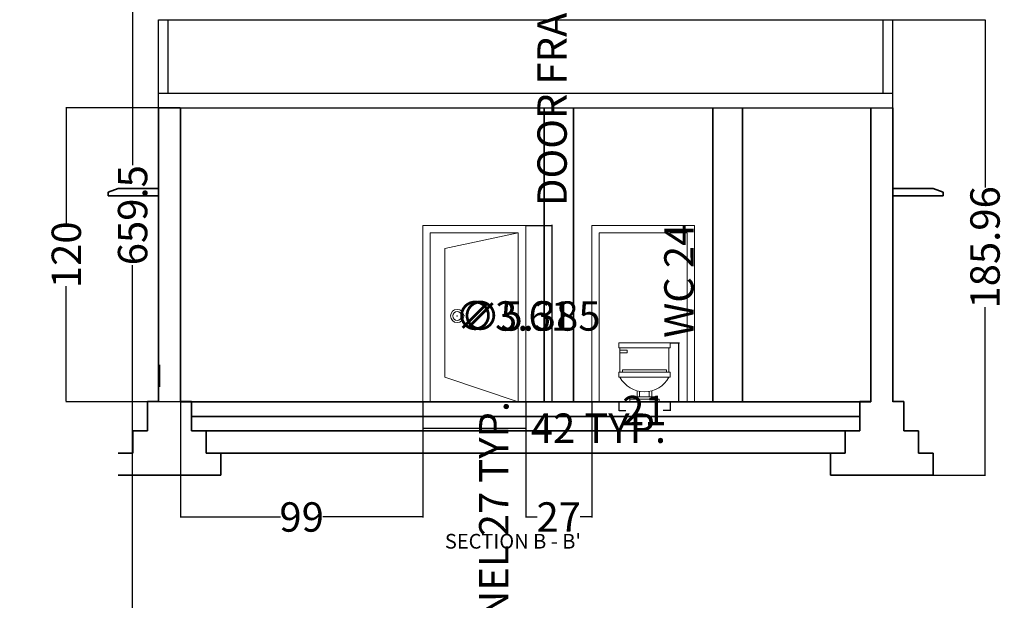
# Model space of a CAD drawing. Units: inches. Extents: x -101 to 786, y 26 to 880.
# Tile 8 of 9: x 379 to 781, y 295 to 532. Entities that reach past the tile are written whole.
import ezdxf

# ---------------------------------------------------------------- set-up
doc = ezdxf.new("R2010")
doc.units = ezdxf.units.IN
doc.header["$MEASUREMENT"] = 0
for name, color, linetype, lineweight in [('A-ANNO-DIMS', 2, 'Continuous', 18), ('A-ANNO-TEXT', 7, 'Continuous', 25), ('A-DOOR', 4, 'Continuous', 20), ('A-FLOR-FIXT', 8, 'Continuous', 18), ('A-ROOF', 7, 'Continuous', 30), ('A-SECT', 7, 'Continuous', 35), ('S-FNDN', 7, 'Continuous', 35)]:
    doc.layers.add(name, color=color, linetype=linetype, lineweight=lineweight)
doc.styles.get("Standard").update_dxf_attribs({"font": 'arial.ttf'})
doc.dimstyles.get("Standard").update_dxf_attribs({"dimtxt": 12, "dimasz": 0.18, "dimexe": 0.18, "dimexo": 0.0625, "dimgap": 0.09, "dimtad": 0, "dimdec": 1, "dimzin": 0, "dimdsep": 46, "dimlunit": 3, "dimtxsty": 'Standard', "dimcen": 0.09, "dimadec": 0, "dimazin": 0, "dimtfac": 1, "dimtdec": 1, "dimtofl": 0, "dimtmove": 0, "dimatfit": 3, "dimfxl": 1, "dimtolj": 1, "dimtzin": 0, "dimarcsym": 0})

# ---------------------------------------------------------------- blocks, each defined once
blk = doc.blocks.new('Toilet - front')
for p, q in [((-10, 22), (-10, 12)), ((-10, 21), (-7, 21)), ((-7, 21), (-7, 20)), ((10, 12), (10, 22)), ((-7, 20), (-10, 20)), ((9, 13), (-9, 13)), ((-9, 13), (-9, 12)), ((9, 12), (9, 13)), ((10.5, 12), (-10.5, 12)), ((-10.5, 10), (-10.5, 12)), ((10.5, 10), (-10.5, 10)), ((10.5, 12), (10.5, 10)), ((-3, 4.4065), (-3, 2)), ((-2, 2), (-2, 4.1658)), ((2, 4.1658), (2, 2)), ((3, 2), (3, 4.4065)), ((4, 2), (-4, 2)), ((-4, 2), (-4, 1)), ((4, 1), (4, 2))]:
    blk.add_line(p, q)
for points in [[(10.5, 22), (10.5, 24), (-10.5, 24), (-10.5, 22)], [(6, 0), (6, 1), (-6, 1), (-6, 0)]]:
    blk.add_lwpolyline(points, close=True)
blk.add_arc((0, 15.3333), 11.3333, 208.0725, 331.9275)
blk = doc.blocks.new('SUNSHADE-SECTION')
for p, q in [((0, 1.5), (4, 3)), ((0, 0), (0, 1.5)), ((20.5, 3), (4, 3)), ((4, 0), (0, 0)), ((20.5, 0), (4, 0))]:
    blk.add_line(p, q)
blk = doc.blocks.new('FOOTING-STEPPED-42')
for p, q in [((12, 30), (12, 18)), ((16.5, 30), (12, 30)), ((30, 30), (25.5, 30)), ((30, 18), (30, 30)), ((12, 18), (6, 18)), ((6, 18), (6, 9)), ((36, 18), (30, 18)), ((36, 9), (36, 18)), ((6, 9), (0, 9)), ((0, 9), (0, 0)), ((42, 9), (36, 9)), ((42, 0), (42, 9)), ((0, 0), (42, 0))]:
    blk.add_line(p, q)
blk = doc.blocks.new('DOOR-FRAME-36x72-SECT')
for points in [[(42, 0), (42, 72), (0, 72), (0, 0)], [(39, 0), (39, 69), (3, 69), (3, 0)]]:
    blk.add_lwpolyline(points)
blk = doc.blocks.new('*D27')
at = {"layer": 'A-ANNO-DIMS', "color": 0, "lineweight": -2, "transparency": 16777216}
for p, q in [((568.37, 262.42), (572.47, 262.42)), ((572.29, 262.42), (572.29, 262.6)), ((572.29, 236.1), (572.29, 262.24)), ((568.37, 235.92), (572.47, 235.92))]:
    blk.add_line(p, q, dxfattribs=at)
at = {"layer": 'A-ANNO-DIMS', "color": 0, "transparency": 16777216}
for points in [[(572.26, 262.24), (572.32, 262.24), (572.29, 262.42)], [(572.26, 236.1), (572.32, 236.1), (572.29, 235.92)]]:
    blk.add_solid(points, dxfattribs=at)
at = {"layer": 'Defpoints', "color": 0, "transparency": 16777216}
for p in [(568.31, 262.42), (572.29, 262.42), (568.31, 235.92)]:
    blk.add_point(p, dxfattribs=at)
at = {"layer": 'A-ANNO-DIMS', "color": 0, "transparency": 16777216, "insert": (572.29, 321.42), "char_height": 12, "attachment_point": 5, "rotation": 90}
blk.add_mtext('\\A1;PANEL 27 TYP.', dxfattribs=at)
blk = doc.blocks.new('*D63')
at = {"layer": 'A-ANNO-DIMS', "color": 0, "lineweight": -2, "transparency": 16777216}
for p, q in [((585.37, 447.92), (596.29, 447.92)), ((596.11, 447.92), (596.11, 448.1)), ((596.11, 376.1), (596.11, 447.74)), ((585.37, 375.92), (596.29, 375.92))]:
    blk.add_line(p, q, dxfattribs=at)
at = {"layer": 'A-ANNO-DIMS', "color": 0, "transparency": 16777216}
for points in [[(596.08, 447.74), (596.14, 447.74), (596.11, 447.92)], [(596.08, 376.1), (596.14, 376.1), (596.11, 375.92)]]:
    blk.add_solid(points, dxfattribs=at)
at = {"layer": 'Defpoints', "color": 0, "transparency": 16777216}
for p in [(585.31, 447.92), (596.11, 447.92), (585.31, 375.92)]:
    blk.add_point(p, dxfattribs=at)
at = {"layer": 'A-ANNO-DIMS', "color": 0, "transparency": 16777216, "insert": (596.11, 536.24), "char_height": 12, "attachment_point": 5, "rotation": 90}
blk.add_mtext('\\A1;DOOR FRAME 72 TYP.', dxfattribs=at)
blk = doc.blocks.new('*D64')
at = {"layer": 'A-ANNO-DIMS', "color": 0, "lineweight": -2, "transparency": 16777216}
for p, q in [((543.31, 375.86), (543.31, 364.94)), ((585.31, 375.86), (585.31, 364.94)), ((543.49, 365.12), (585.13, 365.12)), ((585.31, 365.12), (585.49, 365.12))]:
    blk.add_line(p, q, dxfattribs=at)
at = {"layer": 'A-ANNO-DIMS', "color": 0, "transparency": 16777216}
for points in [[(543.49, 365.15), (543.49, 365.09), (543.31, 365.12)], [(585.13, 365.15), (585.13, 365.09), (585.31, 365.12)]]:
    blk.add_solid(points, dxfattribs=at)
at = {"layer": 'Defpoints', "color": 0, "transparency": 16777216}
for p in [(543.31, 375.92), (585.31, 375.92), (585.31, 365.12)]:
    blk.add_point(p, dxfattribs=at)
at = {"layer": 'A-ANNO-DIMS', "color": 0, "transparency": 16777216, "insert": (615.03, 365.12), "char_height": 12, "attachment_point": 5}
blk.add_mtext('\\A1;42 TYP.', dxfattribs=at)
blk = doc.blocks.new('*D77')
at = {"layer": 'A-ANNO-DIMS', "color": 0, "lineweight": -2, "transparency": 16777216}
for p, q in [((644.37, 399.92), (648.09, 399.92)), ((647.91, 399.92), (647.91, 400.1)), ((647.91, 376.1), (647.91, 399.74)), ((644.37, 375.92), (648.09, 375.92))]:
    blk.add_line(p, q, dxfattribs=at)
at = {"layer": 'A-ANNO-DIMS', "color": 0, "transparency": 16777216}
for points in [[(647.88, 399.74), (647.94, 399.74), (647.91, 399.92)], [(647.88, 376.1), (647.94, 376.1), (647.91, 375.92)]]:
    blk.add_solid(points, dxfattribs=at)
at = {"layer": 'Defpoints', "color": 0, "transparency": 16777216}
for p in [(644.31, 399.92), (647.91, 399.92), (644.31, 375.92)]:
    blk.add_point(p, dxfattribs=at)
at = {"layer": 'A-ANNO-DIMS', "color": 0, "transparency": 16777216, "insert": (647.91, 425.3), "char_height": 12, "attachment_point": 5, "rotation": 90}
blk.add_mtext('\\A1;WC 24', dxfattribs=at)
blk = doc.blocks.new('*D78')
at = {"layer": 'A-ANNO-DIMS', "color": 0, "lineweight": -2, "transparency": 16777216}
for p, q in [((623.31, 375.86), (623.31, 372.14)), ((644.31, 375.86), (644.31, 372.14)), ((623.49, 372.32), (626.18, 372.32)), ((644.13, 372.32), (641.44, 372.32))]:
    blk.add_line(p, q, dxfattribs=at)
at = {"layer": 'A-ANNO-DIMS', "color": 0, "transparency": 16777216}
for points in [[(623.49, 372.35), (623.49, 372.29), (623.31, 372.32)], [(644.13, 372.35), (644.13, 372.29), (644.31, 372.32)]]:
    blk.add_solid(points, dxfattribs=at)
at = {"layer": 'Defpoints', "color": 0, "transparency": 16777216}
for p in [(623.31, 375.92), (644.31, 375.92), (644.31, 372.32)]:
    blk.add_point(p, dxfattribs=at)
at = {"layer": 'A-ANNO-DIMS', "color": 0, "transparency": 16777216, "insert": (633.81, 372.32), "char_height": 12, "attachment_point": 5}
blk.add_mtext('\\A1;21', dxfattribs=at)
blk = doc.blocks.new('*D80')
at = {"layer": 'A-ANNO-DIMS', "color": 0, "lineweight": -2, "transparency": 16777216}
for p, q in [((323.57, 781.8), (424.94, 781.8)), ((424.76, 781.62), (424.76, 472.49)), ((424.76, 122.52), (424.76, 431.66)), ((323.57, 122.34), (424.94, 122.34))]:
    blk.add_line(p, q, dxfattribs=at)
at = {"layer": 'A-ANNO-DIMS', "color": 0, "transparency": 16777216}
for points in [[(424.73, 781.62), (424.79, 781.62), (424.76, 781.8)], [(424.73, 122.52), (424.79, 122.52), (424.76, 122.34)]]:
    blk.add_solid(points, dxfattribs=at)
at = {"layer": 'Defpoints', "color": 0, "transparency": 16777216}
for p in [(323.51, 781.8), (424.76, 781.8), (323.51, 122.34)]:
    blk.add_point(p, dxfattribs=at)
at = {"layer": 'A-ANNO-DIMS', "color": 0, "transparency": 16777216, "insert": (424.76, 452.07), "char_height": 12, "attachment_point": 5, "rotation": 90}
blk.add_mtext('\\A1;659.5', dxfattribs=at)
blk = doc.blocks.new('*D125')
at = {"layer": 'A-ANNO-DIMS', "color": 0, "lineweight": -2, "transparency": 16777216}
for p, q in [((735.37, 531.92), (773.12, 531.92)), ((772.94, 531.74), (772.94, 463.37)), ((772.94, 346.14), (772.94, 414.51)), ((751.88, 345.96), (773.12, 345.96))]:
    blk.add_line(p, q, dxfattribs=at)
at = {"layer": 'A-ANNO-DIMS', "color": 0, "transparency": 16777216}
for points in [[(772.91, 531.74), (772.97, 531.74), (772.94, 531.92)], [(772.91, 346.14), (772.97, 346.14), (772.94, 345.96)]]:
    blk.add_solid(points, dxfattribs=at)
at = {"layer": 'Defpoints', "color": 0, "transparency": 16777216}
for p in [(735.31, 531.92), (772.94, 531.92), (751.82, 345.96)]:
    blk.add_point(p, dxfattribs=at)
at = {"layer": 'A-ANNO-DIMS', "color": 0, "transparency": 16777216, "insert": (772.94, 438.94), "char_height": 12, "attachment_point": 5, "rotation": 90}
blk.add_mtext('\\A1;185.96', dxfattribs=at)
blk = doc.blocks.new('*D126')
at = {"layer": 'A-ANNO-DIMS', "color": 0, "lineweight": -2, "transparency": 16777216}
for p, q in [((444.25, 495.92), (397.5, 495.92)), ((397.68, 495.74), (397.68, 448.69)), ((397.68, 376.1), (397.68, 423.16)), ((444.25, 375.92), (397.5, 375.92))]:
    blk.add_line(p, q, dxfattribs=at)
at = {"layer": 'A-ANNO-DIMS', "color": 0, "transparency": 16777216}
for points in [[(397.65, 495.74), (397.71, 495.74), (397.68, 495.92)], [(397.65, 376.1), (397.71, 376.1), (397.68, 375.92)]]:
    blk.add_solid(points, dxfattribs=at)
at = {"layer": 'Defpoints', "color": 0, "transparency": 16777216}
for p in [(397.68, 495.92), (444.31, 495.92), (444.31, 375.92)]:
    blk.add_point(p, dxfattribs=at)
at = {"layer": 'A-ANNO-DIMS', "color": 0, "transparency": 16777216, "insert": (397.68, 435.92), "char_height": 12, "attachment_point": 5, "rotation": 90}
blk.add_mtext('\\A1;120', dxfattribs=at)
blk = doc.blocks.new('*D127')
at = {"layer": 'A-ANNO-DIMS', "color": 0, "lineweight": -2, "transparency": 16777216}
for p, q in [((444.31, 375.86), (444.31, 328.66)), ((543.31, 375.86), (543.31, 328.66)), ((444.49, 328.84), (485.11, 328.84)), ((543.13, 328.84), (502.51, 328.84))]:
    blk.add_line(p, q, dxfattribs=at)
at = {"layer": 'A-ANNO-DIMS', "color": 0, "transparency": 16777216}
for points in [[(444.49, 328.87), (444.49, 328.81), (444.31, 328.84)], [(543.13, 328.87), (543.13, 328.81), (543.31, 328.84)]]:
    blk.add_solid(points, dxfattribs=at)
at = {"layer": 'Defpoints', "color": 0, "transparency": 16777216}
for p in [(444.31, 375.92), (543.31, 375.92), (543.31, 328.84)]:
    blk.add_point(p, dxfattribs=at)
at = {"layer": 'A-ANNO-DIMS', "color": 0, "transparency": 16777216, "insert": (493.81, 328.84), "char_height": 12, "attachment_point": 5}
blk.add_mtext('\\A1;99', dxfattribs=at)
blk = doc.blocks.new('*D128')
at = {"layer": 'A-ANNO-DIMS', "color": 0, "lineweight": -2, "transparency": 16777216}
for p, q in [((585.31, 375.86), (585.31, 328.66)), ((612.31, 375.86), (612.31, 328.66)), ((585.49, 328.84), (590.02, 328.84)), ((612.13, 328.84), (607.6, 328.84))]:
    blk.add_line(p, q, dxfattribs=at)
at = {"layer": 'A-ANNO-DIMS', "color": 0, "transparency": 16777216}
for points in [[(585.49, 328.87), (585.49, 328.81), (585.31, 328.84)], [(612.13, 328.87), (612.13, 328.81), (612.31, 328.84)]]:
    blk.add_solid(points, dxfattribs=at)
at = {"layer": 'Defpoints', "color": 0, "transparency": 16777216}
for p in [(585.31, 375.92), (612.31, 375.92), (612.31, 328.84)]:
    blk.add_point(p, dxfattribs=at)
at = {"layer": 'A-ANNO-DIMS', "color": 0, "transparency": 16777216, "insert": (598.81, 328.84), "char_height": 12, "attachment_point": 5}
blk.add_mtext('\\A1;27', dxfattribs=at)
blk = doc.blocks.new('*D139')
at = {"layer": 'A-ANNO-DIMS', "color": 0, "lineweight": -2, "transparency": 16777216}
for p, q in [((557.22, 410.92), (557.4, 410.92)), ((557.31, 410.83), (557.31, 411.01)), ((560.36, 410.92), (560.18, 410.92))]:
    blk.add_line(p, q, dxfattribs=at)
at = {"layer": 'A-ANNO-DIMS', "color": 0, "transparency": 16777216}
blk.add_solid([(560.18, 410.95), (560.18, 410.89), (560, 410.92)], dxfattribs=at)
at = {"layer": 'Defpoints', "color": 0, "transparency": 16777216}
for p in [(554.62, 410.92), (560, 410.92)]:
    blk.add_point(p, dxfattribs=at)
at = {"layer": 'A-ANNO-DIMS', "color": 0, "transparency": 16777216, "insert": (587.27, 410.93), "char_height": 12, "attachment_point": 5, "rotation": 0.0045}
blk.add_mtext('\\A1;∅5.385', dxfattribs=at)
blk = doc.blocks.new('*D140')
at = {"layer": 'A-ANNO-DIMS', "color": 0, "lineweight": -2, "transparency": 16777216}
for p, q in [((557.22, 410.92), (557.4, 410.92)), ((557.31, 410.83), (557.31, 411.01)), ((559.47, 410.92), (559.29, 410.92))]:
    blk.add_line(p, q, dxfattribs=at)
at = {"layer": 'A-ANNO-DIMS', "color": 0, "transparency": 16777216}
blk.add_solid([(559.29, 410.95), (559.29, 410.89), (559.11, 410.92)], dxfattribs=at)
at = {"layer": 'Defpoints', "color": 0, "transparency": 16777216}
for p in [(555.51, 410.92), (559.11, 410.92)]:
    blk.add_point(p, dxfattribs=at)
at = {"layer": 'A-ANNO-DIMS', "color": 0, "transparency": 16777216, "insert": (580.52, 410.93), "char_height": 12, "attachment_point": 5, "rotation": 0.0067}
blk.add_mtext('\\A1;∅3.61', dxfattribs=at)

msp = doc.modelspace()

# ---------------------------------------------------------------- linework, layer by layer
at = {"layer": 'A-DOOR'}
for p, q in [((543.3117, 447.9238), (585.3117, 447.9238)), ((582.3117, 444.9238), (552.3117, 438.4238)), ((552.3117, 438.4238), (552.3117, 385.9238)), ((552.3117, 385.9238), (582.3117, 375.9238))]:
    msp.add_line(p, q, dxfattribs=at)
for radius in [2.6926, 2.6926, 1.8028]:
    msp.add_circle((557.3117, 410.9238), radius, dxfattribs=at)
at = {"layer": 'A-ROOF'}
for p, q in [((435.3117, 531.9238), (735.3117, 531.9238)), ((435.3117, 495.9238), (435.3117, 531.9238)), ((439.3117, 501.9238), (439.3117, 531.9238)), ((731.3117, 501.9238), (731.3117, 531.9238)), ((735.3117, 495.9238), (735.3117, 531.9238)), ((435.3117, 501.9238), (735.3117, 501.9238)), ((435.3117, 495.9238), (735.3117, 495.9238))]:
    msp.add_line(p, q, dxfattribs=at)
at = {"layer": 'A-SECT'}
for p, q in [((435.3117, 375.9238), (435.3117, 495.9238)), ((444.3117, 375.9238), (444.3117, 495.9238)), ((592.8117, 375.9238), (592.8117, 495.9238)), ((604.8117, 375.9238), (604.8117, 495.9238)), ((661.8117, 455.4238), (661.8117, 495.9238)), ((673.8117, 455.4238), (673.8117, 495.9238)), ((726.3117, 375.9238), (726.3117, 495.9238)), ((735.3117, 375.9238), (735.3117, 495.9238)), ((435.8069, 390.9606), (435.8069, 381.9606)), ((444.3117, 375.9238), (726.3117, 375.9238))]:
    msp.add_line(p, q, dxfattribs=at)
for points in [[(604.8117, 455.4238), (604.8117, 375.9238)], [(661.8117, 375.9238), (661.8117, 455.4238)], [(673.8117, 375.9238), (673.8117, 455.4238)]]:
    msp.add_lwpolyline(points, dxfattribs=at)
at = {"layer": 'S-FNDN'}
for p, q in [((435.3117, 375.9606), (430.8069, 375.9606)), ((430.8069, 375.9606), (430.8069, 363.9606)), ((448.8069, 375.9606), (444.3117, 375.9606)), ((448.8069, 363.9606), (448.8069, 375.9606)), ((448.8069, 369.9238), (721.8166, 369.9238)), ((430.8069, 363.9606), (424.8069, 363.9606)), ((424.8069, 363.9606), (424.8069, 354.9606)), ((454.8069, 363.9606), (448.8069, 363.9606)), ((454.8069, 354.9606), (454.8069, 363.9606)), ((454.8069, 363.9606), (715.8166, 363.9606)), ((424.8069, 354.9606), (418.8069, 354.9606)), ((460.8069, 354.9606), (454.8069, 354.9606)), ((460.8069, 345.9606), (460.8069, 354.9606)), ((460.8069, 354.9606), (709.8166, 354.9606)), ((418.8069, 345.9606), (460.8069, 345.9606))]:
    msp.add_line(p, q, dxfattribs=at)

# ---------------------------------------------------------------- block references
at = {"layer": 'A-DOOR'}
for p in [(543.312, 375.924), (612.312, 375.924)]:
    msp.add_blockref('DOOR-FRAME-36x72-SECT', p, dxfattribs=at)
at = {"layer": 'A-FLOR-FIXT'}
msp.add_blockref('Toilet - front', (633.8117, 375.9238), dxfattribs=at)
at = {"layer": 'A-SECT'}
msp.add_blockref('SUNSHADE-SECTION', (414.807, 459.961), dxfattribs=at)
at = {"layer": 'A-SECT', "extrusion": (0, 0, -1), "zscale": -1}
msp.add_blockref('SUNSHADE-SECTION', (-755.8165, 459.961), dxfattribs=at)
at = {"layer": 'S-FNDN', "extrusion": (0, 0, -1), "zscale": -1}
msp.add_blockref('FOOTING-STEPPED-42', (-751.8165, 345.961), dxfattribs=at)

# ---------------------------------------------------------------- texts
at = {"layer": 'A-ANNO-TEXT'}
msp.add_text("SECTION B - B'", height=6, dxfattribs=at).set_placement((552.3117, 315.9238))

# ---------------------------------------------------------------- dimensions: what is measured, and where the dimension line sits
at = {"layer": 'A-ANNO-DIMS'}
for base, p1, p2, override, picture, middle in [((424.7579, 781.8033), (323.5071, 122.3446), (323.5071, 781.8033), {"dimdec": 1, "dimlfac": 1, "dimrnd": 0, "dimzin": 0, "dimdsep": 46, "dimlunit": 2}, '*D80', (424.7579, 452.0739)), ((772.9416, 531.9238), (751.8166, 345.9606), (735.3117, 531.9238), {"dimdec": 2, "dimlfac": 1, "dimrnd": 0, "dimzin": 0, "dimdsep": 46, "dimlunit": 2}, '*D125', (772.9416, 438.9422)), ((397.6819, 495.9238), (444.3117, 375.9238), (444.3117, 495.9238), {"dimdec": 0, "dimlfac": 1, "dimrnd": 0, "dimzin": 0, "dimdsep": 46, "dimlunit": 2}, '*D126', (397.6819, 435.9238))]:
    dim = msp.add_linear_dim(base=base, p1=p1, p2=p2, angle=90, dimstyle='Standard', override=override, dxfattribs=at)
    dim.commit()
    dim.dimension.update_dxf_attribs({"geometry": picture, "text_midpoint": middle})
for base, p1, p2, text, picture, middle in [((596.1117, 447.9238), (585.3117, 375.9238), (585.3117, 447.9238), 'DOOR FRAME <> TYP.', '*D63', (596.1117, 536.2415)), ((647.9117, 399.9238), (644.3117, 375.9238), (644.3117, 399.9238), 'WC <>', '*D77', (647.9117, 425.3029)), ((572.2867420758, 262.4237895654), (568.3117420758, 235.9237895654), (568.3117420758, 262.4237895654), 'PANEL <> TYP.', '*D27', (572.2867420758, 321.4168454999))]:
    dim = msp.add_linear_dim(base=base, p1=p1, p2=p2, angle=90, text=text, dimstyle='Standard', override={"dimdec": 0, "dimlfac": 1, "dimrnd": 0, "dimzin": 0, "dimdsep": 46, "dimlunit": 2}, dxfattribs=at)
    dim.commit()
    dim.dimension.update_dxf_attribs({"geometry": picture, "text_midpoint": middle})
dim = msp.add_diameter_dim_2p(p1=(554.6192, 410.9236), p2=(560.0043, 410.924), dimstyle='Standard', override={"dimdec": 3, "dimlfac": 1, "dimrnd": 0, "dimzin": 0, "dimdsep": 46, "dimlunit": 2}, dxfattribs=at)
dim.commit()
dim.dimension.update_dxf_attribs({"geometry": '*D139', "text_midpoint": (587.2742, 410.9261), "dimtype": 163})
dim = msp.add_diameter_dim_2p(p1=(555.509, 410.9236), p2=(559.1145, 410.924), dimstyle='Standard', override={"dimdec": 2, "dimlfac": 1, "dimrnd": 0, "dimzin": 0, "dimdsep": 46, "dimlunit": 2}, dxfattribs=at)
dim.commit()
dim.dimension.update_dxf_attribs({"geometry": '*D140', "text_midpoint": (580.5195, 410.9265)})
dim = msp.add_linear_dim(base=(585.3117, 365.1238), p1=(543.3117, 375.9238), p2=(585.3117, 375.9238), text='<> TYP.', dimstyle='Standard', override={"dimdec": 0, "dimlfac": 1, "dimrnd": 0, "dimzin": 0, "dimdsep": 46, "dimlunit": 2}, dxfattribs=at)
dim.commit()
dim.dimension.update_dxf_attribs({"geometry": '*D64', "text_midpoint": (615.0292, 365.1238)})
for base, p1, p2, picture, middle in [((644.3117, 372.3238), (623.3117, 375.9238), (644.3117, 375.9238), '*D78', (633.8117, 372.3238)), ((543.3117, 328.8356), (444.3117, 375.9238), (543.3117, 375.9238), '*D127', (493.8117, 328.8356)), ((612.3117, 328.8356), (585.3117, 375.9238), (612.3117, 375.9238), '*D128', (598.8117, 328.8356))]:
    dim = msp.add_linear_dim(base=base, p1=p1, p2=p2, dimstyle='Standard', override={"dimdec": 0, "dimlfac": 1, "dimrnd": 0, "dimzin": 0, "dimdsep": 46, "dimlunit": 2}, dxfattribs=at)
    dim.commit()
    dim.dimension.update_dxf_attribs({"geometry": picture, "text_midpoint": middle})

doc.saveas('drawing.dxf')
